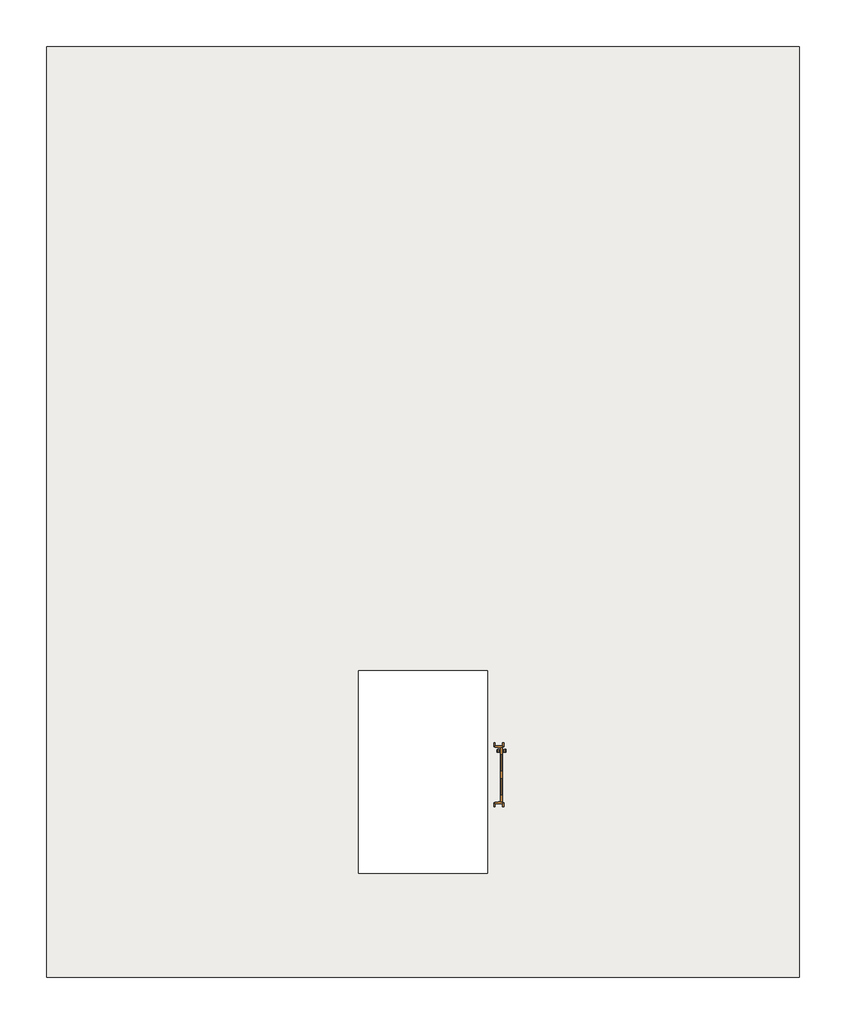
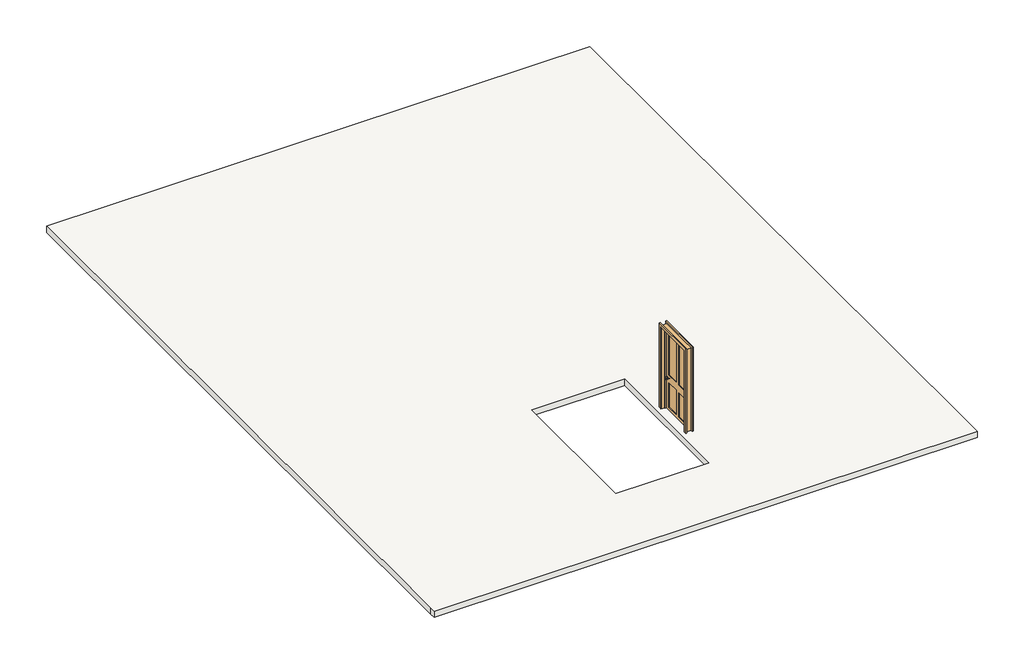
# One storey: 1 door, 1 roof.
"""IFC4 building model written with IfcOpenShell, lengths in millimetres."""

from ifc_helpers import new_model, si_unit, frame, origin, place, context, project, spatial, polyline, outline, extrude, transform, mapped, element, save
from components import door_68a706ac

model = new_model("IFC4")

# Units and contexts
model_context = context("Model", 3, world=origin())
ifc_project = project(units=[si_unit("LENGTHUNIT", "METRE", prefix="MILLI")], contexts=[model_context])

# Site, building, storey
site = spatial("IfcSite", under=ifc_project)
building = spatial("IfcBuilding", under=site)
storey = spatial("IfcBuildingStorey", under=building, Elevation=6400.8)

# Door
placement = place(None, origin())
door_shape = door_68a706ac(model_context)
element("IfcDoor", 1, ObjectType="Door-Interior-Single-4_Panel-Wood : 36\" x 84\"", at=placement, inside=storey, context=model_context, shape_type="MappedRepresentation", body=[
    mapped(door_shape, transform((-8278.5021954, -3327.2640253, 6400.8), x_axis=(0.0, -1.0, 0.0), y_axis=(1.0, 0.0, 0.0), z_axis=(0.0, 0.0, 1.0))),
])

# Roof
element("IfcRoof", 2, ObjectType="slab 1 6\"", at=placement, inside=storey, context=model_context, shape_type="SweptSolid", body=[
    extrude(outline(polyline([(-15776.2646954, 8733.1272103), (-3303.2771954, 8733.1272103), (-3303.2771954, -6379.8727897), (-3303.2771954, -6684.6727897), (-15776.2646954, -6684.6727897), (-15776.2646954, -6532.2727897), (-15776.2646954, 8733.1272103)]), holes=[polyline([(-10605.7771954, -4957.4727897), (-8472.1771954, -4957.4727897), (-8472.1771954, -1604.6727897), (-10605.7771954, -1604.6727897), (-10605.7771954, -4957.4727897)])]), frame((0.0, 0.0, 6400.8), z_axis=(0.0, 0.0, 1.0), x_axis=(1.0, 0.0, 0.0)), (0.0, 0.0, 1.0), 152.4),
])

save(model, "model.ifc")

# Revit data of these elements
# Type "Door-Interior-Single-4_Panel-Wood : 36\" x 84\""
#   Type Mark = "10"
#   Assembly Code = "C1020300"
#   Analytic Construction = "Wooden"
#   Top Rail = 0' - 4 11/16"
#   Thickness = 0' - 1 3/8"
#   Thermal Resistance (R) = 2.5876 (h·ft²·°F)/BTU
#   Swing Angle [instance default] = 90.00°
#   Stiles = 0' - 4 3/4"
#   Rough Width = 3' - 2"
#   Rough Height = 7' - 1"
#   Mullion = 0' - 4 1/2"
#   Lock Rail = 0' - 7 1/2"
#   Height = 7' - 0"
#   Width = 3' - 0"
#   Heat Transfer Coefficient (U) = 0.3865 BTU/(h·ft²·°F)
#   Bottom Rail = 0' - 9 1/8"
#   Trim Material = Cherry
#   Panel Material = Cherry
#   Frame Material = Cherry
#   Door Handle Material = Aluminum
#   Visual Light Transmittance = 0
#   Solar Heat Gain Coefficient = 0
#   Wall Closure = (empty or 0)
#   Function = (empty or 0)
# Type "slab 1 6\""
#   Assembly Code = "B1020"
#   Layers, outside or top first: 0' - 6" "slab colour" (function 1)
# Element 1 (IfcDoor, "Door-Interior-Single-4_Panel-Wood : 36\" x 84\"")
#   Swing Angle = 90.00°
#   Phase Created = New Construction
#   Materials on its faces: "Cherry", "Aluminum"
# Element 2 (IfcRoof, "slab 1 6\"")
#   built-in parameter 1001705 = 21.5 (stored number, unit not read)
#   built-in parameter 1001710 = 33615
#   Phase Created = New Construction
#   Materials on its faces: "Porcelain, Linen", "slab colour", "Porcelain, Ivory"
# Materials
#   "Cherry": class "Wood", colour RGB 226 177 128, transparency 0, Description = "Prunus Serotina", Cost = 0
#   "Aluminum": class "Metal", colour RGB 247 247 247, transparency 0, Description = "Aluminum 6061", Cost = 0
#   "slab colour": class "Generic", colour RGB 120 120 120, transparency 0, Cost = 0
#   "Porcelain, Linen": class "Ceramic", colour RGB 249 239 230, transparency 0, Description = "Porcelain, linen", Cost = 0
#   "Porcelain, Ivory": class "Ceramic", colour RGB 247 247 239, transparency 0, Description = "Porcelain, ivory", Cost = 0
